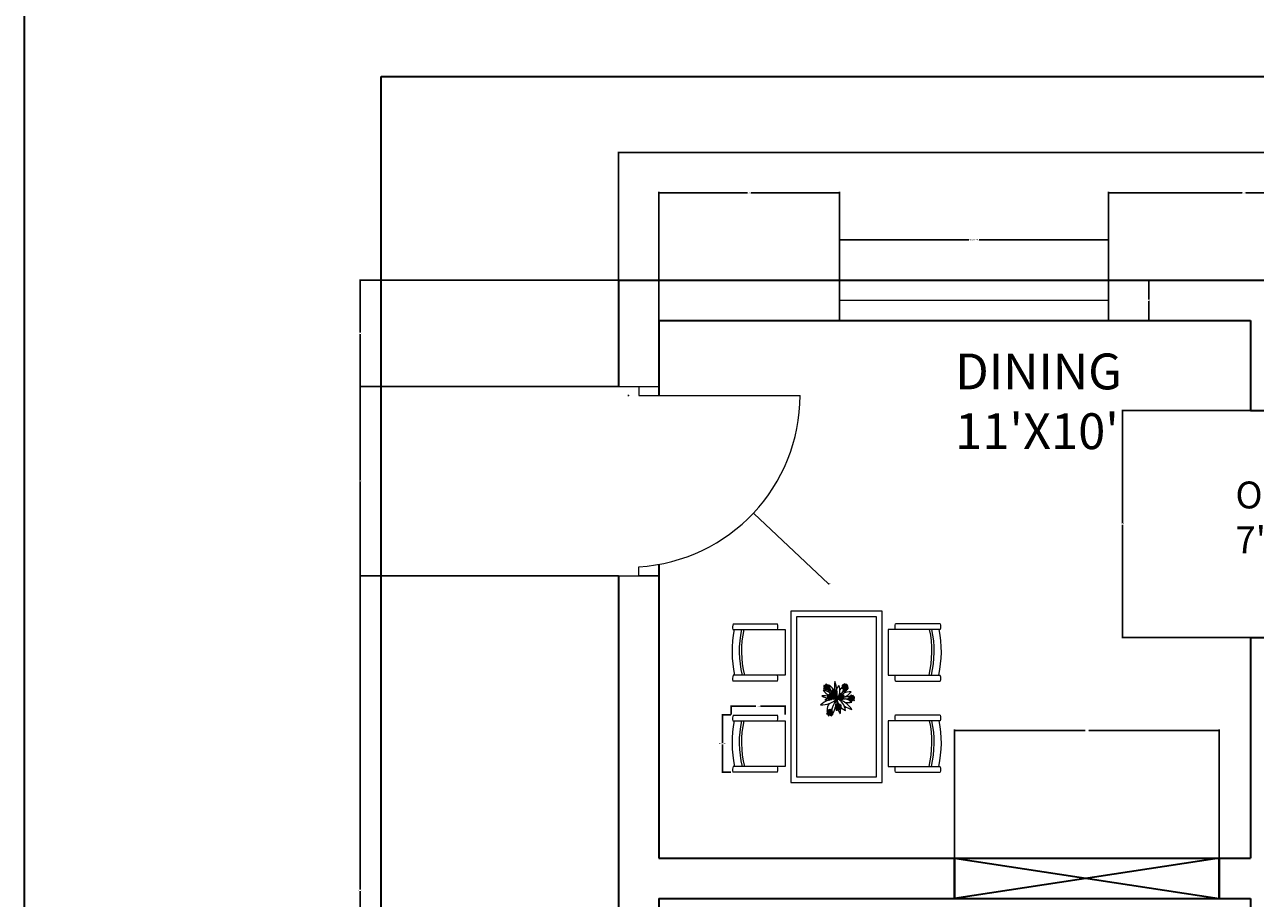
# Model space of a CAD drawing. Units: inches. Extents: x 1976 to 2558, y -977 to 2909.
# Tile 5 of 8: x 1976 to 2251, y 2245 to 2441. Entities that reach past the tile are written whole.
import ezdxf

# ---------------------------------------------------------------- set-up
doc = ezdxf.new("R2010")
doc.units = ezdxf.units.IN
for name, color, linetype, lineweight in [('A-ANNO-DIMS', 2, 'Continuous', 18), ('A-ANNO-TTLB', 7, 'Continuous', 35), ('A-AREA-IDEN', 7, 'Continuous', 18), ('A-DOOR', 3, 'Continuous', 18), ('A-FURN', 8, 'Continuous', 13), ('A-GLAZ', 4, 'Continuous', 18), ('A-WALL', 7, 'Continuous', 35)]:
    doc.layers.add(name, color=color, linetype=linetype, lineweight=lineweight)
doc.styles.get("Standard").update_dxf_attribs({"font": 'arial.ttf'})
doc.dimstyles.get("Standard").update_dxf_attribs({"dimtxt": 0.18, "dimasz": 0.18, "dimexe": 0.18, "dimexo": 0.0625, "dimgap": 0.09, "dimtad": 0, "dimtih": 1, "dimtoh": 1, "dimdec": 4, "dimzin": 0, "dimdsep": 46, "dimtxsty": 'Standard', "dimcen": 0.09, "dimadec": 0, "dimazin": 0, "dimtfac": 1, "dimtdec": 4, "dimtofl": 0, "dimtmove": 0, "dimatfit": 3, "dimfxl": 1, "dimtolj": 1, "dimtzin": 0, "dimarcsym": 0})

# ---------------------------------------------------------------- blocks, each defined once
blk = doc.blocks.new('CHAIR-DINING')
for p, q in [((0.21, 11.47), (11.84, 11.47)), ((0.23, 12.75), (10.16, 12.75)), ((11.84, 11.47), (11.84, 1.28)), ((10.17, 0), (0.21, 0)), ((11.84, 1.28), (0.23, 1.28))]:
    blk.add_line(p, q)
for centre, radius, start, end in [((25.08, 6.69), 25.08, 168.9982, 192.4562), ((2.1, 12.08), 1.98, 160.4535, 197.9116), ((25.42, 6.69), 23.81, 168.4012, 193.1346), ((25.42, 6.69), 23.3, 168.1438, 193.4274), ((8.28, 12.1), 1.98, 342.2774, 19.7376), ((2.1, 0.6), 1.98, 160.2624, 197.7226), ((8.28, 0.6), 1.98, 342.2774, 19.7376)]:
    blk.add_arc(centre, radius, start, end)
blk = doc.blocks.new('WIN-60-PLAN')
for p, q in [((4.5, 60), (0, 60)), ((0, 60), (9, 60)), ((4.5, 0), (4.5, 60)), ((0, 0), (9, 0)), ((9, 0), (4.5, 0))]:
    blk.add_line(p, q)
blk = doc.blocks.new('*D9')
at = {"layer": 'A-ANNO-DIMS', "color": 0, "lineweight": -2, "transparency": 16777216}
for p, q in [((2133.49, 2286.43), (2131.45, 2286.43)), ((2131.63, 2286.25), (2131.63, 2280.23)), ((2131.63, 2273.84), (2131.63, 2279.86)), ((2133.49, 2273.66), (2131.45, 2273.66))]:
    blk.add_line(p, q, dxfattribs=at)
at = {"layer": 'A-ANNO-DIMS', "color": 0, "transparency": 16777216}
for points in [[(2131.6, 2286.25), (2131.66, 2286.25), (2131.63, 2286.43)], [(2131.6, 2273.84), (2131.66, 2273.84), (2131.63, 2273.66)]]:
    blk.add_solid(points, dxfattribs=at)
at = {"layer": 'Defpoints', "color": 0, "transparency": 16777216}
for p in [(2131.63, 2286.43), (2133.55, 2286.43), (2133.55, 2273.66)]:
    blk.add_point(p, dxfattribs=at)
at = {"layer": 'A-ANNO-DIMS', "color": 0, "transparency": 16777216, "insert": (2131.63, 2280.05), "char_height": 0.18, "attachment_point": 5}
blk.add_mtext('\\A1;CHAIR 13 TYP.', dxfattribs=at)
blk = doc.blocks.new('*D10')
at = {"layer": 'A-ANNO-DIMS', "color": 0, "lineweight": -2, "transparency": 16777216}
for p, q in [((2133.55, 2286.49), (2133.55, 2288.53)), ((2133.73, 2288.35), (2139.05, 2288.35)), ((2145.4, 2288.35), (2140.09, 2288.35)), ((2145.58, 2286.49), (2145.58, 2288.53))]:
    blk.add_line(p, q, dxfattribs=at)
at = {"layer": 'A-ANNO-DIMS', "color": 0, "transparency": 16777216}
for points in [[(2133.73, 2288.38), (2133.73, 2288.32), (2133.55, 2288.35)], [(2145.4, 2288.38), (2145.4, 2288.32), (2145.58, 2288.35)]]:
    blk.add_solid(points, dxfattribs=at)
at = {"layer": 'Defpoints', "color": 0, "transparency": 16777216}
for p in [(2145.58, 2288.35), (2133.55, 2286.43), (2145.58, 2286.43)]:
    blk.add_point(p, dxfattribs=at)
at = {"layer": 'A-ANNO-DIMS', "color": 0, "transparency": 16777216, "insert": (2139.57, 2288.35), "char_height": 0.18, "attachment_point": 5}
blk.add_mtext('\\A1;12 TYP.', dxfattribs=at)
blk = doc.blocks.new('*D11')
at = {"layer": 'A-ANNO-DIMS', "color": 0, "lineweight": -2, "transparency": 16777216}
for p, q in [((2157.76, 2383.54), (2157.76, 2392.66)), ((2157.94, 2392.48), (2186.64, 2392.48)), ((2217.58, 2392.48), (2188.88, 2392.48)), ((2217.76, 2383.54), (2217.76, 2392.66))]:
    blk.add_line(p, q, dxfattribs=at)
at = {"layer": 'A-ANNO-DIMS', "color": 0, "transparency": 16777216}
for points in [[(2157.94, 2392.51), (2157.94, 2392.45), (2157.76, 2392.48)], [(2217.58, 2392.51), (2217.58, 2392.45), (2217.76, 2392.48)]]:
    blk.add_solid(points, dxfattribs=at)
at = {"layer": 'Defpoints', "color": 0, "transparency": 16777216}
for p in [(2217.76, 2392.48), (2157.76, 2383.48), (2217.76, 2383.48)]:
    blk.add_point(p, dxfattribs=at)
at = {"layer": 'A-ANNO-DIMS', "color": 0, "transparency": 16777216, "insert": (2187.76, 2392.48), "char_height": 0.18, "attachment_point": 5}
blk.add_mtext('\\A1;WINDOW 60 TYP.', dxfattribs=at)
blk = doc.blocks.new('*D12')
at = {"layer": 'A-ANNO-DIMS', "color": 0, "lineweight": -2, "transparency": 16777216}
for p, q in [((2217.82, 2383.48), (2226.94, 2383.48)), ((2226.76, 2383.3), (2226.76, 2379.16)), ((2226.76, 2374.66), (2226.76, 2378.8)), ((2217.82, 2374.48), (2226.94, 2374.48))]:
    blk.add_line(p, q, dxfattribs=at)
at = {"layer": 'A-ANNO-DIMS', "color": 0, "transparency": 16777216}
for points in [[(2226.73, 2383.3), (2226.79, 2383.3), (2226.76, 2383.48)], [(2226.73, 2374.66), (2226.79, 2374.66), (2226.76, 2374.48)]]:
    blk.add_solid(points, dxfattribs=at)
at = {"layer": 'Defpoints', "color": 0, "transparency": 16777216}
for p in [(2217.76, 2383.48), (2217.76, 2374.48), (2226.76, 2374.48)]:
    blk.add_point(p, dxfattribs=at)
at = {"layer": 'A-ANNO-DIMS', "color": 0, "transparency": 16777216, "insert": (2226.76, 2378.98), "char_height": 0.18, "attachment_point": 5}
blk.add_mtext('\\A1;9 TYP.', dxfattribs=at)
blk = doc.blocks.new('*D23')
at = {"layer": 'A-ANNO-DIMS', "color": 0, "lineweight": -2, "transparency": 16777216}
for p, q in [((2108.44, 2383.54), (2108.44, 2412.16)), ((2108.62, 2411.98), (2256.65, 2411.98)), ((2405.26, 2411.98), (2257.23, 2411.98)), ((2405.44, 2383.54), (2405.44, 2412.16))]:
    blk.add_line(p, q, dxfattribs=at)
at = {"layer": 'A-ANNO-DIMS', "color": 0, "transparency": 16777216}
for points in [[(2108.62, 2412.01), (2108.62, 2411.95), (2108.44, 2411.98)], [(2405.26, 2412.01), (2405.26, 2411.95), (2405.44, 2411.98)]]:
    blk.add_solid(points, dxfattribs=at)
at = {"layer": 'Defpoints', "color": 0, "transparency": 16777216}
for p in [(2405.44, 2411.98), (2108.44, 2383.48), (2405.44, 2383.48)]:
    blk.add_point(p, dxfattribs=at)
at = {"layer": 'A-ANNO-DIMS', "color": 0, "transparency": 16777216, "insert": (2256.94, 2411.98), "char_height": 0.18, "attachment_point": 5}
blk.add_mtext('\\A1;297', dxfattribs=at)
blk = doc.blocks.new('*D28')
at = {"layer": 'A-ANNO-DIMS', "color": 0, "lineweight": -2, "transparency": 16777216}
for p, q in [((2117.44, 2374.54), (2117.44, 2403.16)), ((2117.62, 2402.98), (2137.2, 2402.98)), ((2157.58, 2402.98), (2137.99, 2402.98)), ((2157.76, 2374.54), (2157.76, 2403.16))]:
    blk.add_line(p, q, dxfattribs=at)
at = {"layer": 'A-ANNO-DIMS', "color": 0, "transparency": 16777216}
for points in [[(2117.62, 2403.01), (2117.62, 2402.95), (2117.44, 2402.98)], [(2157.58, 2403.01), (2157.58, 2402.95), (2157.76, 2402.98)]]:
    blk.add_solid(points, dxfattribs=at)
at = {"layer": 'Defpoints', "color": 0, "transparency": 16777216}
for p in [(2157.76, 2402.98), (2117.44, 2374.48), (2157.76, 2374.48)]:
    blk.add_point(p, dxfattribs=at)
at = {"layer": 'A-ANNO-DIMS', "color": 0, "transparency": 16777216, "insert": (2137.6, 2402.98), "char_height": 0.18, "attachment_point": 5}
blk.add_mtext('\\A1;40.32', dxfattribs=at)
blk = doc.blocks.new('*D29')
at = {"layer": 'A-ANNO-DIMS', "color": 0, "lineweight": -2, "transparency": 16777216}
for p, q in [((2217.76, 2374.54), (2217.76, 2403.16)), ((2217.94, 2402.98), (2247.63, 2402.98)), ((2278.11, 2402.98), (2248.42, 2402.98)), ((2278.29, 2374.54), (2278.29, 2403.16))]:
    blk.add_line(p, q, dxfattribs=at)
at = {"layer": 'A-ANNO-DIMS', "color": 0, "transparency": 16777216}
for points in [[(2217.94, 2403.01), (2217.94, 2402.95), (2217.76, 2402.98)], [(2278.11, 2403.01), (2278.11, 2402.95), (2278.29, 2402.98)]]:
    blk.add_solid(points, dxfattribs=at)
at = {"layer": 'Defpoints', "color": 0, "transparency": 16777216}
for p in [(2278.29, 2402.98), (2217.76, 2374.48), (2278.29, 2374.48)]:
    blk.add_point(p, dxfattribs=at)
at = {"layer": 'A-ANNO-DIMS', "color": 0, "transparency": 16777216, "insert": (2248.02, 2402.98), "char_height": 0.18, "attachment_point": 5}
blk.add_mtext('\\A1;60.53', dxfattribs=at)
blk = doc.blocks.new('*D33')
at = {"layer": 'A-ANNO-DIMS', "color": 0, "lineweight": -2, "transparency": 16777216}
for p, q in [((2108.38, 2383.48), (2050.58, 2383.48)), ((2050.76, 2383.3), (2050.76, 2371.8)), ((2050.76, 2359.93), (2050.76, 2371.43)), ((2108.38, 2359.75), (2050.58, 2359.75))]:
    blk.add_line(p, q, dxfattribs=at)
at = {"layer": 'A-ANNO-DIMS', "color": 0, "transparency": 16777216}
for points in [[(2050.73, 2383.3), (2050.79, 2383.3), (2050.76, 2383.48)], [(2050.73, 2359.93), (2050.79, 2359.93), (2050.76, 2359.75)]]:
    blk.add_solid(points, dxfattribs=at)
at = {"layer": 'Defpoints', "color": 0, "transparency": 16777216}
for p in [(2108.44, 2383.48), (2050.76, 2359.75), (2108.44, 2359.75)]:
    blk.add_point(p, dxfattribs=at)
at = {"layer": 'A-ANNO-DIMS', "color": 0, "transparency": 16777216, "insert": (2050.76, 2371.61), "char_height": 0.18, "attachment_point": 5}
blk.add_mtext('\\A1;23.73', dxfattribs=at)
blk = doc.blocks.new('*D34')
at = {"layer": 'A-ANNO-DIMS', "color": 0, "lineweight": -2, "transparency": 16777216}
for p, q in [((2108.38, 2359.75), (2050.58, 2359.75)), ((2050.76, 2359.57), (2050.76, 2338.8)), ((2050.76, 2317.68), (2050.76, 2338.44)), ((2108.38, 2317.5), (2050.58, 2317.5))]:
    blk.add_line(p, q, dxfattribs=at)
at = {"layer": 'A-ANNO-DIMS', "color": 0, "transparency": 16777216}
for points in [[(2050.73, 2359.57), (2050.79, 2359.57), (2050.76, 2359.75)], [(2050.73, 2317.68), (2050.79, 2317.68), (2050.76, 2317.5)]]:
    blk.add_solid(points, dxfattribs=at)
at = {"layer": 'Defpoints', "color": 0, "transparency": 16777216}
for p in [(2108.44, 2359.75), (2050.76, 2317.5), (2108.44, 2317.5)]:
    blk.add_point(p, dxfattribs=at)
at = {"layer": 'A-ANNO-DIMS', "color": 0, "transparency": 16777216, "insert": (2050.76, 2338.62), "char_height": 0.18, "attachment_point": 5}
blk.add_mtext('\\A1;42.25', dxfattribs=at)
blk = doc.blocks.new('*D35')
at = {"layer": 'A-ANNO-DIMS', "color": 0, "lineweight": -2, "transparency": 16777216}
for p, q in [((2108.38, 2317.5), (2050.58, 2317.5)), ((2050.76, 2317.32), (2050.76, 2247.46)), ((2050.76, 2177.24), (2050.76, 2247.1)), ((2108.38, 2177.06), (2050.58, 2177.06))]:
    blk.add_line(p, q, dxfattribs=at)
at = {"layer": 'A-ANNO-DIMS', "color": 0, "transparency": 16777216}
for points in [[(2050.73, 2317.32), (2050.79, 2317.32), (2050.76, 2317.5)], [(2050.73, 2177.24), (2050.79, 2177.24), (2050.76, 2177.06)]]:
    blk.add_solid(points, dxfattribs=at)
at = {"layer": 'Defpoints', "color": 0, "transparency": 16777216}
for p in [(2108.44, 2317.5), (2050.76, 2177.06), (2108.44, 2177.06)]:
    blk.add_point(p, dxfattribs=at)
at = {"layer": 'A-ANNO-DIMS', "color": 0, "transparency": 16777216, "insert": (2050.76, 2247.28), "char_height": 0.18, "attachment_point": 5}
blk.add_mtext('\\A1;140.44', dxfattribs=at)
blk = doc.blocks.new('*D49')
at = {"layer": 'A-ANNO-DIMS', "color": 0, "lineweight": -2, "transparency": 16777216}
for p, q in [((2249.38, 2354.4), (2220.76, 2354.4)), ((2220.94, 2354.22), (2220.94, 2329.25)), ((2220.94, 2303.92), (2220.94, 2328.89)), ((2249.38, 2303.74), (2220.76, 2303.74))]:
    blk.add_line(p, q, dxfattribs=at)
at = {"layer": 'A-ANNO-DIMS', "color": 0, "transparency": 16777216}
for points in [[(2220.91, 2354.22), (2220.97, 2354.22), (2220.94, 2354.4)], [(2220.91, 2303.92), (2220.97, 2303.92), (2220.94, 2303.74)]]:
    blk.add_solid(points, dxfattribs=at)
at = {"layer": 'Defpoints', "color": 0, "transparency": 16777216}
for p in [(2220.94, 2354.4), (2249.44, 2354.4), (2249.44, 2303.74)]:
    blk.add_point(p, dxfattribs=at)
at = {"layer": 'A-ANNO-DIMS', "color": 0, "transparency": 16777216, "insert": (2220.94, 2329.07), "char_height": 0.18, "attachment_point": 5}
blk.add_mtext('\\A1;50.67', dxfattribs=at)
blk = doc.blocks.new('*D50')
at = {"layer": 'A-ANNO-DIMS', "color": 0, "lineweight": -2, "transparency": 16777216}
for p, q in [((2183.44, 2254.54), (2183.44, 2283.16)), ((2183.62, 2282.98), (2212.58, 2282.98)), ((2242.33, 2282.98), (2213.37, 2282.98)), ((2242.51, 2254.54), (2242.51, 2283.16))]:
    blk.add_line(p, q, dxfattribs=at)
at = {"layer": 'A-ANNO-DIMS', "color": 0, "transparency": 16777216}
for points in [[(2183.62, 2283.01), (2183.62, 2282.95), (2183.44, 2282.98)], [(2242.33, 2283.01), (2242.33, 2282.95), (2242.51, 2282.98)]]:
    blk.add_solid(points, dxfattribs=at)
at = {"layer": 'Defpoints', "color": 0, "transparency": 16777216}
for p in [(2242.51, 2282.98), (2183.44, 2254.48), (2242.51, 2254.48)]:
    blk.add_point(p, dxfattribs=at)
at = {"layer": 'A-ANNO-DIMS', "color": 0, "transparency": 16777216, "insert": (2212.97, 2282.98), "char_height": 0.18, "attachment_point": 5}
blk.add_mtext('\\A1;59.07', dxfattribs=at)
blk = doc.blocks.new('*D89')
at = {"layer": 'A-ANNO-DIMS', "color": 0, "lineweight": -2, "transparency": 16777216}
for p, q in [((2110.53, 2357.75), (2110.71, 2357.75)), ((2110.62, 2357.66), (2110.62, 2357.84)), ((2155.27, 2315.73), (2138.65, 2331.36)), ((2155.45, 2315.73), (2155.27, 2315.73))]:
    blk.add_line(p, q, dxfattribs=at)
at = {"layer": 'A-ANNO-DIMS', "color": 0, "transparency": 16777216}
blk.add_solid([(2138.67, 2331.38), (2138.63, 2331.34), (2138.52, 2331.48)], dxfattribs=at)
at = {"layer": 'Defpoints', "color": 0, "transparency": 16777216}
for p in [(2110.62, 2357.75), (2138.52, 2331.48)]:
    blk.add_point(p, dxfattribs=at)
at = {"layer": 'A-ANNO-DIMS', "color": 0, "transparency": 16777216, "insert": (2155.92, 2315.73), "char_height": 0.18, "attachment_point": 5}
blk.add_mtext('\\A1;R38.32', dxfattribs=at)

msp = doc.modelspace()

# ---------------------------------------------------------------- linework, layer by layer
at = {"layer": 'A-ANNO-TTLB'}
for points in [[(1975.8545, 2909.3429), (2557.9168, 2909.3429), (2557.9168, 1747.8598), (1975.8545, 1747.8598)], [(2055.4343, 2428.9091), (2450.0007, 2428.9091), (2450.0007, 1815.3916), (2055.4343, 1815.3916)]]:
    msp.add_lwpolyline(points, close=True, dxfattribs=at)
at = {"layer": 'A-DOOR'}
for p, q in [((2108.4385, 2359.7476), (2117.4385, 2359.7476)), ((2112.9385, 2359.7476), (2112.9385, 2357.7476)), ((2112.9385, 2357.7476), (2148.9385, 2357.7476)), ((2112.9385, 2317.4977), (2112.9385, 2319.4977)), ((2108.4385, 2317.4977), (2117.4385, 2317.4977)), ((2117.4385, 2317.4977), (2112.9385, 2317.4977))]:
    msp.add_line(p, q, dxfattribs=at)
msp.add_arc((2110.6183, 2357.7476), 38.3202, 273.471228, 0, dxfattribs=at)
at = {"layer": 'A-FURN'}
for points in [[(2167.272, 2309.6099), (2146.8785, 2309.6099), (2146.8785, 2271.372), (2167.272, 2271.372)], [(2165.9974, 2308.3353), (2148.1531, 2308.3353), (2148.1531, 2272.6466), (2165.9974, 2272.6466)]]:
    msp.add_lwpolyline(points, close=True, dxfattribs=at)
for centre, radius, start, end in [((2164.1832, 2292.9107), 7.5857, 172.300876, 189.713934), ((2149.6339, 2291.0822), 7.5857, 352.300876, 22.025549), ((2158.1534, 2295.1251), 5.1574, 217.808391, 258.794638), ((2153.0765, 2286.9043), 5.1574, 60.607319, 78.794638), ((2154.169, 2293.3715), 1.0315, 269.156448, 313.437642), ((2154.8631, 2291.5911), 1.0315, 89.156448, 133.437642), ((2154.3081, 2291.3787), 1.3683, 65.373219, 94.46089), ((2154.7718, 2293.9866), 1.3683, 245.373219, 274.46089), ((2155.0787, 2293.6343), 1.0315, 217.808391, 258.794638), ((2154.0633, 2291.9902), 1.0315, 60.607319, 78.794638), ((2154.687, 2291.6856), 0.9563, 78.462149, 111.54354), ((2154.5271, 2293.512), 0.9563, 258.462149, 268.298065), ((2155.632, 2293.808), 1.4049, 211.28949, 237.552058), ((2153.6777, 2291.8929), 1.4049, 31.28949, 57.552058), ((2154.9539, 2292.1195), 0.5087, 145.613299, 182.653681), ((2154.3701, 2292.599), 0.5087, 278.552081, 306.302355), ((2154.0572, 2292.5582), 0.8235, 4.476283, 53.763425), ((2155.3651, 2293.2868), 0.8235, 184.476283, 205.355726), ((2156.0281, 2291.8073), 1.4095, 144.666489, 178.965307), ((2153.469, 2292.648), 1.4095, 324.666489, 343.955925), ((2156.2847, 2293.1915), 1.5171, 172.300876, 189.713934), ((2153.3748, 2292.8258), 1.5171, 352.300876, 22.025549), ((2155.6455, 2292.3211), 0.8243, 158.556067, 197.254243), ((2154.091, 2292.378), 0.8243, 338.556067, 17.254243), ((2155.3702, 2292.8464), 0.5405, 138.054662, 156.71607), ((2154.4763, 2292.9838), 0.5405, 318.054662, 24.46723), ((2153.8722, 2294.2269), 1.8938, 302.089724, 323.743755), ((2156.4053, 2291.5025), 1.8938, 122.089724, 143.743755), ((2155.4004, 2290.8199), 1.8767, 82.537441, 106.153056), ((2155.122, 2294.4833), 1.8767, 262.537441, 286.153056), ((2155.5237, 2292.6892), 0.6489, 185.896009, 246.101931), ((2154.6154, 2292.0293), 0.6489, 5.896009, 66.101931), ((2154.5562, 2291.4603), 1.206, 34.273745, 74.509726), ((2155.8019, 2292.4719), 0.9358, 195.544227, 214.461724), ((2151.1486, 2286.4178), 7.0243, 31.28949, 57.552058), ((2160.9199, 2295.9936), 7.0243, 211.28949, 237.552058), ((2155.6877, 2292.5572), 0.812, 124.966344, 145.814561), ((2154.1067, 2292.093), 0.9358, 350.741507, 11.174689), ((2154.4129, 2293.288), 0.812, 331.307439, 355.385611), ((2155.4951, 2292.1452), 0.7799, 88.595575, 113.612418), ((2155.8748, 2293.3017), 1.206, 236.312373, 254.509726), ((2154.8974, 2293.4022), 0.7799, 293.448679, 322.265702), ((2155.3799, 2293.2756), 0.8235, 258.712866, 281.757983), ((2155.0461, 2291.8162), 0.8235, 52.470844, 74.980876), ((2159.5852, 2293.3872), 4.1177, 184.476283, 205.355726), ((2153.0461, 2289.7446), 4.1177, 4.476283, 53.763425), ((2157.095, 2290.9992), 1.5171, 172.300876, 189.713934), ((2154.1851, 2290.6335), 1.5171, 352.300876, 22.025549), ((2156.4836, 2290.3886), 1.0315, 89.156448, 133.437642), ((2155.7896, 2292.169), 1.0315, 269.156448, 313.437642), ((2155.9287, 2290.1762), 1.3683, 65.373219, 94.46089), ((2156.3924, 2292.7841), 1.3683, 245.373219, 274.46089), ((2155.6839, 2290.7877), 1.0315, 60.607319, 78.794638), ((2156.6993, 2292.4318), 1.0315, 217.808391, 258.794638), ((2156.3076, 2290.483), 0.9563, 78.462149, 111.54354), ((2156.1477, 2292.3094), 0.9563, 258.462149, 268.298065), ((2157.2526, 2292.6055), 1.4049, 211.28949, 237.552058), ((2155.2983, 2290.6903), 1.4049, 31.28949, 57.552058), ((2156.5745, 2290.9169), 0.5087, 145.613299, 182.653681), ((2156.9856, 2292.0842), 0.8235, 184.476283, 205.355726), ((2155.6778, 2291.3557), 0.8235, 4.476283, 53.763425), ((2157.6487, 2290.6048), 1.4095, 144.666489, 178.965307), ((2157.9052, 2291.9889), 1.5171, 172.300876, 189.713934), ((2154.9954, 2291.6232), 1.5171, 352.300876, 22.025549), ((2157.2661, 2291.1186), 0.8243, 158.556067, 197.254243), ((2155.7116, 2291.1755), 0.8243, 338.556067, 17.254243), ((2156.9908, 2291.6438), 0.5405, 138.054662, 156.71607), ((2156.0968, 2291.7813), 0.5405, 318.054662, 24.46723), ((2155.4928, 2293.0244), 1.8938, 302.089724, 323.743755), ((2158.0259, 2290.3), 1.8938, 122.089724, 143.743755), ((2157.0209, 2289.6174), 1.8767, 82.537441, 106.153056), ((2156.7426, 2293.2808), 1.8767, 262.537441, 286.153056), ((2157.1443, 2291.4866), 0.6489, 185.896009, 246.101931), ((2156.236, 2290.8267), 0.6489, 5.896009, 66.101931), ((2156.1767, 2290.2578), 1.206, 34.273745, 74.509726), ((2157.3082, 2291.3546), 0.812, 124.966344, 145.814561), ((2156.0335, 2292.0854), 0.812, 331.307439, 355.385611), ((2157.1157, 2290.9426), 0.7799, 88.595575, 113.612418), ((2157.4954, 2292.0991), 1.206, 236.312373, 254.509726), ((2156.5179, 2292.1997), 0.7799, 293.448679, 322.265702), ((2157.0005, 2292.0731), 0.8235, 258.712866, 281.757983), ((2156.6666, 2290.6137), 0.8235, 52.470844, 74.980876), ((2159.611, 2291.1852), 2.7025, 138.054662, 156.71607), ((2155.1411, 2291.8723), 2.7025, 318.054662, 24.46723), ((2152.1209, 2298.088), 9.4688, 302.089724, 323.743755), ((2164.7866, 2284.4661), 9.4688, 122.089724, 143.743755), ((2157.2984, 2290.4303), 0.8235, 4.476283, 53.763425), ((2158.6062, 2291.1588), 0.8235, 184.476283, 205.355726), ((2161.1982, 2289.7393), 4.0602, 124.966344, 145.814561), ((2159.5258, 2291.0635), 1.5171, 172.300876, 189.713934), ((2156.6159, 2290.6978), 1.5171, 352.300876, 22.025549), ((2158.6114, 2290.7184), 0.5405, 138.054662, 156.71607), ((2157.7174, 2290.8558), 0.5405, 318.054662, 24.46723), ((2158.9145, 2291.6609), 1.0315, 89.156448, 133.437642), ((2158.2205, 2293.4412), 1.0315, 269.156448, 313.437642), ((2158.3595, 2291.4484), 1.3683, 65.373219, 94.46089), ((2158.8233, 2294.0564), 1.3683, 245.373219, 274.46089), ((2158.9288, 2290.4292), 0.812, 124.966344, 145.814561), ((2159.1301, 2293.7041), 1.0315, 217.808391, 258.794638), ((2158.1147, 2292.0599), 1.0315, 60.607319, 78.794638), ((2157.654, 2291.16), 0.812, 331.307439, 355.385611), ((2154.8243, 2293.3932), 4.0602, 331.307439, 355.385611), ((2158.7384, 2291.7553), 0.9563, 78.462149, 111.54354), ((2158.5785, 2293.5817), 0.9563, 258.462149, 268.298065), ((2159.6834, 2293.8778), 1.4049, 211.28949, 237.552058), ((2157.7292, 2291.9626), 1.4049, 31.28949, 57.552058), ((2159.0053, 2292.1892), 0.5087, 145.613299, 182.653681), ((2158.4215, 2292.6687), 0.5087, 278.552081, 306.302355), ((2159.4165, 2293.3565), 0.8235, 184.476283, 205.355726), ((2158.1087, 2292.628), 0.8235, 4.476283, 53.763425), ((2160.0796, 2291.8771), 1.4095, 144.666489, 178.965307), ((2157.5204, 2292.7177), 1.4095, 324.666489, 343.955925), ((2160.2353, 2287.6793), 3.8997, 88.595575, 113.612418), ((2157.2468, 2293.9645), 3.8997, 293.448679, 322.265702), ((2160.3361, 2293.2612), 1.5171, 172.300876, 189.713934), ((2157.4262, 2292.8955), 1.5171, 352.300876, 22.025549), ((2159.6969, 2292.3909), 0.8243, 158.556067, 197.254243), ((2158.1425, 2292.4477), 0.8243, 338.556067, 17.254243), ((2159.4216, 2292.9161), 0.5405, 138.054662, 156.71607), ((2158.5277, 2293.0535), 0.5405, 318.054662, 24.46723), ((2157.9236, 2294.2967), 1.8938, 302.089724, 323.743755), ((2160.4568, 2291.5723), 1.8938, 122.089724, 143.743755), ((2159.4518, 2290.8896), 1.8767, 82.537441, 106.153056), ((2159.1734, 2294.553), 1.8767, 262.537441, 286.153056), ((2159.5751, 2292.7589), 0.6489, 185.896009, 246.101931), ((2158.6668, 2292.099), 0.6489, 5.896009, 66.101931), ((2158.6076, 2291.5301), 1.206, 34.273745, 74.509726), ((2159.8533, 2292.5417), 0.9358, 195.544227, 214.461724), ((2159.7391, 2292.6269), 0.812, 124.966344, 145.814561), ((2158.1581, 2292.1627), 0.9358, 350.741507, 11.174689), ((2158.4643, 2293.3577), 0.812, 331.307439, 355.385611), ((2159.5465, 2292.2149), 0.7799, 88.595575, 113.612418), ((2159.9263, 2293.3714), 1.206, 236.312373, 254.509726), ((2158.9488, 2293.472), 0.7799, 293.448679, 322.265702), ((2159.4314, 2293.3453), 0.8235, 258.712866, 281.757983), ((2159.0975, 2291.886), 0.8235, 52.470844, 74.980876), ((2157.0753, 2284.909), 5.1575, 89.156448, 133.437642), ((2153.6051, 2293.8109), 5.1575, 269.156448, 313.437642), ((2154.3003, 2283.8468), 6.8414, 65.373219, 94.46089), ((2156.6191, 2296.8866), 6.8414, 245.373219, 274.46089), ((2156.1949, 2285.3813), 4.7813, 78.462149, 111.54354), ((2155.3955, 2294.5132), 4.7813, 258.462149, 268.298065), ((2155.6734, 2289.3988), 1.0315, 89.156448, 133.437642), ((2154.9793, 2291.1792), 1.0315, 269.156448, 313.437642), ((2157.5294, 2287.5508), 2.5435, 145.613299, 182.653681), ((2155.1184, 2289.1864), 1.3683, 65.373219, 94.46089), ((2155.5821, 2291.7944), 1.3683, 245.373219, 274.46089), ((2155.889, 2291.4421), 1.0315, 217.808391, 258.794638), ((2154.8736, 2289.7979), 1.0315, 60.607319, 78.794638), ((2155.4973, 2289.4933), 0.9563, 78.462149, 111.54354), ((2155.3374, 2291.3197), 0.9563, 258.462149, 268.298065), ((2156.4423, 2291.6158), 1.4049, 211.28949, 237.552058), ((2154.488, 2289.7006), 1.4049, 31.28949, 57.552058), ((2155.7642, 2289.9272), 0.5087, 145.613299, 182.653681), ((2155.1804, 2290.4067), 0.5087, 278.552081, 306.302355), ((2154.8675, 2290.366), 0.8235, 4.476283, 53.763425), ((2156.1754, 2291.0945), 0.8235, 184.476283, 205.355726), ((2156.8384, 2289.6151), 1.4095, 144.666489, 178.965307), ((2154.2793, 2290.4557), 1.4095, 324.666489, 343.955925), ((2156.4558, 2290.1289), 0.8243, 158.556067, 197.254243), ((2154.9013, 2290.1857), 0.8243, 338.556067, 17.254243), ((2156.1805, 2290.6541), 0.5405, 138.054662, 156.71607), ((2155.2865, 2290.7915), 0.5405, 318.054662, 24.46723), ((2154.6825, 2292.0347), 1.8938, 302.089724, 323.743755), ((2157.2156, 2289.3103), 1.8938, 122.089724, 143.743755), ((2156.2106, 2288.6276), 1.8767, 82.537441, 106.153056), ((2155.9323, 2292.291), 1.8767, 262.537441, 286.153056), ((2156.334, 2290.4969), 0.6489, 185.896009, 246.101931), ((2155.4257, 2289.837), 0.6489, 5.896009, 66.101931), ((2155.3665, 2289.2681), 1.206, 34.273745, 74.509726), ((2156.6122, 2290.2797), 0.9358, 195.544227, 214.461724), ((2156.498, 2290.3649), 0.812, 124.966344, 145.814561), ((2154.917, 2289.9007), 0.9358, 350.741507, 11.174689), ((2162.9006, 2285.9901), 7.0476, 144.666489, 178.965307), ((2155.2232, 2291.0957), 0.812, 331.307439, 355.385611), ((2156.3054, 2289.9529), 0.7799, 88.595575, 113.612418), ((2156.6851, 2291.1094), 1.206, 236.312373, 254.509726), ((2155.7077, 2291.2099), 0.7799, 293.448679, 322.265702), ((2156.1902, 2291.0833), 0.8235, 258.712866, 281.757983), ((2155.9907, 2291.3964), 0.5087, 278.552081, 306.302355), ((2155.8564, 2289.624), 0.8235, 52.470844, 74.980876), ((2155.0896, 2291.4454), 1.4095, 324.666489, 343.955925), ((2157.4225, 2291.2694), 0.9358, 195.544227, 214.461724), ((2155.7272, 2290.8904), 0.9358, 350.741507, 11.174689), ((2156.874, 2287.0313), 1.3683, 65.373219, 94.46089), ((2157.3377, 2289.6392), 1.3683, 245.373219, 274.46089), ((2156.6292, 2287.6428), 1.0315, 60.607319, 78.794638), ((2157.6446, 2289.2869), 1.0315, 217.808391, 258.794638), ((2160.9874, 2288.5591), 4.1216, 158.556067, 197.254243), ((2158.1979, 2289.4606), 1.4049, 211.28949, 237.552058), ((2156.2436, 2287.5455), 1.4049, 31.28949, 57.552058), ((2153.2151, 2288.8434), 4.1216, 338.556067, 17.254243), ((2156.6231, 2288.2108), 0.8235, 4.476283, 53.763425), ((2157.931, 2288.9394), 0.8235, 184.476283, 205.355726), ((2159.7617, 2281.053), 9.3834, 82.537441, 106.153056), ((2158.3699, 2299.3699), 9.3834, 262.537441, 286.153056), ((2160.3784, 2290.3992), 3.2443, 185.896009, 246.101931), ((2155.8369, 2287.0997), 3.2443, 5.896009, 66.101931), ((2155.5407, 2284.2551), 6.0299, 34.273745, 74.509726), ((2158.8506, 2288.8441), 1.5171, 172.300876, 189.713934), ((2155.9407, 2288.4784), 1.5171, 352.300876, 22.025549), ((2158.1042, 2289.4631), 1.0315, 89.156448, 133.437642), ((2157.4102, 2291.2435), 1.0315, 269.156448, 313.437642), ((2157.9361, 2288.499), 0.5405, 138.054662, 156.71607), ((2157.5492, 2289.2507), 1.3683, 65.373219, 94.46089), ((2158.013, 2291.8587), 1.3683, 245.373219, 274.46089), ((2157.0422, 2288.6364), 0.5405, 318.054662, 24.46723), ((2156.4381, 2289.8795), 1.8938, 302.089724, 323.743755), ((2158.9712, 2287.1551), 1.8938, 122.089724, 143.743755), ((2157.9663, 2286.4725), 1.8767, 82.537441, 106.153056), ((2157.6879, 2290.1359), 1.8767, 262.537441, 286.153056), ((2158.3198, 2291.5064), 1.0315, 217.808391, 258.794638), ((2157.3045, 2289.8622), 1.0315, 60.607319, 78.794638), ((2157.9281, 2289.5576), 0.9563, 78.462149, 111.54354), ((2157.7683, 2291.384), 0.9563, 258.462149, 268.298065), ((2158.2536, 2288.2098), 0.812, 124.966344, 145.814561), ((2158.8731, 2291.6801), 1.4049, 211.28949, 237.552058), ((2156.9189, 2289.7649), 1.4049, 31.28949, 57.552058), ((2158.195, 2289.9915), 0.5087, 145.613299, 182.653681), ((2157.6113, 2290.471), 0.5087, 278.552081, 306.302355), ((2156.9788, 2288.9406), 0.812, 331.307439, 355.385611), ((2158.061, 2287.7978), 0.7799, 88.595575, 113.612418), ((2157.4633, 2289.0548), 0.7799, 293.448679, 322.265702), ((2159.2693, 2289.6794), 1.4095, 144.666489, 178.965307), ((2156.7101, 2290.52), 1.4095, 324.666489, 343.955925), ((2158.8867, 2290.1932), 0.8243, 158.556067, 197.254243), ((2157.3322, 2290.25), 0.8243, 338.556067, 17.254243), ((2159.6465, 2289.3746), 1.8938, 122.089724, 143.743755), ((2157.1134, 2292.099), 1.8938, 302.089724, 323.743755), ((2158.6415, 2288.6919), 1.8767, 82.537441, 106.153056), ((2158.3631, 2292.3553), 1.8767, 262.537441, 286.153056), ((2157.7973, 2289.3324), 1.206, 34.273745, 74.509726), ((2158.7648, 2290.5612), 0.6489, 185.896009, 246.101931), ((2157.8565, 2289.9013), 0.6489, 5.896009, 66.101931), ((2159.043, 2290.344), 0.9358, 195.544227, 214.461724), ((2157.3478, 2289.965), 0.9358, 350.741507, 11.174689), ((2158.7362, 2290.0172), 0.7799, 88.595575, 113.612418), ((2159.116, 2291.1737), 1.206, 236.312373, 254.509726), ((2158.1385, 2291.2742), 0.7799, 293.448679, 322.265702), ((2158.6211, 2291.1476), 0.8235, 258.712866, 281.757983), ((2158.2872, 2289.6883), 0.8235, 52.470844, 74.980876), ((2162.134, 2293.4617), 6.0299, 236.312373, 254.509726), ((2159.6595, 2293.3315), 4.1177, 258.712866, 281.757983), ((2157.9903, 2286.0347), 4.1177, 52.470844, 74.980876), ((2160.4, 2289.129), 1.0315, 89.156448, 133.437642), ((2159.706, 2290.9094), 1.0315, 269.156448, 313.437642), ((2159.845, 2288.9166), 1.3683, 65.373219, 94.46089), ((2160.3088, 2291.5245), 1.3683, 245.373219, 274.46089), ((2160.6157, 2291.1722), 1.0315, 217.808391, 258.794638), ((2159.6003, 2289.5281), 1.0315, 60.607319, 78.794638), ((2160.2239, 2289.2235), 0.9563, 78.462149, 111.54354), ((2160.0641, 2291.0498), 0.9563, 258.462149, 268.298065), ((2159.2147, 2289.4308), 1.4049, 31.28949, 57.552058), ((2161.169, 2291.3459), 1.4049, 211.28949, 237.552058), ((2160.4909, 2289.6574), 0.5087, 145.613299, 182.653681), ((2159.9071, 2290.1368), 0.5087, 278.552081, 306.302355), ((2159.5942, 2290.0961), 0.8235, 4.476283, 53.763425), ((2160.902, 2290.8246), 0.8235, 184.476283, 205.355726), ((2161.5651, 2289.3452), 1.4095, 144.666489, 178.965307), ((2159.0059, 2290.1858), 1.4095, 324.666489, 343.955925), ((2161.8216, 2290.7293), 1.5171, 172.300876, 189.713934), ((2158.9118, 2290.3636), 1.5171, 352.300876, 22.025549), ((2161.1825, 2289.859), 0.8243, 158.556067, 197.254243), ((2159.628, 2289.9159), 0.8243, 338.556067, 17.254243), ((2160.9072, 2290.3842), 0.5405, 138.054662, 156.71607), ((2160.0132, 2290.5217), 0.5405, 318.054662, 24.46723), ((2161.9423, 2289.0404), 1.8938, 122.089724, 143.743755), ((2159.4092, 2291.7648), 1.8938, 302.089724, 323.743755), ((2160.9373, 2288.3578), 1.8767, 82.537441, 106.153056), ((2160.6589, 2292.0212), 1.8767, 262.537441, 286.153056), ((2161.0606, 2290.227), 0.6489, 185.896009, 246.101931), ((2160.1523, 2289.5671), 0.6489, 5.896009, 66.101931), ((2160.0931, 2288.9982), 1.206, 34.273745, 74.509726), ((2161.3388, 2290.0098), 0.9358, 195.544227, 214.461724), ((2161.2246, 2290.0951), 0.812, 124.966344, 145.814561), ((2159.6436, 2289.6309), 0.9358, 350.741507, 11.174689), ((2159.9498, 2290.8258), 0.812, 331.307439, 355.385611), ((2161.032, 2289.6831), 0.7799, 88.595575, 113.612418), ((2161.4118, 2290.8395), 1.206, 236.312373, 254.509726), ((2160.4343, 2290.9401), 0.7799, 293.448679, 322.265702), ((2160.9169, 2290.8135), 0.8235, 258.712866, 281.757983), ((2160.583, 2289.3541), 0.8235, 52.470844, 74.980876), ((2155.5383, 2285.9243), 1.0315, 89.156448, 133.437642), ((2154.8443, 2287.7047), 1.0315, 269.156448, 313.437642), ((2154.9833, 2285.7119), 1.3683, 65.373219, 94.46089), ((2155.4471, 2288.3199), 1.3683, 245.373219, 274.46089), ((2155.7539, 2287.9676), 1.0315, 217.808391, 258.794638), ((2154.7386, 2286.3234), 1.0315, 60.607319, 78.794638), ((2154.6105, 2289.9482), 2.5435, 278.552081, 306.302355), ((2155.3622, 2286.0188), 0.9563, 78.462149, 111.54354), ((2155.2024, 2287.8452), 0.9563, 258.462149, 268.298065), ((2156.3072, 2288.1413), 1.4049, 211.28949, 237.552058), ((2154.353, 2286.2261), 1.4049, 31.28949, 57.552058), ((2155.6291, 2286.4527), 0.5087, 145.613299, 182.653681), ((2155.0454, 2286.9322), 0.5087, 278.552081, 306.302355), ((2154.7325, 2286.8915), 0.8235, 4.476283, 53.763425), ((2156.0403, 2287.62), 0.8235, 184.476283, 205.355726), ((2156.7034, 2286.1406), 1.4095, 144.666489, 178.965307), ((2154.1442, 2286.9812), 1.4095, 324.666489, 343.955925), ((2156.9599, 2287.5247), 1.5171, 172.300876, 189.713934), ((2154.05, 2287.159), 1.5171, 352.300876, 22.025549), ((2156.3208, 2286.6544), 0.8243, 158.556067, 197.254243), ((2154.7663, 2286.7112), 0.8243, 338.556067, 17.254243), ((2156.0455, 2287.1796), 0.5405, 138.054662, 156.71607), ((2155.1515, 2287.317), 0.5405, 318.054662, 24.46723), ((2154.5474, 2288.5602), 1.8938, 302.089724, 323.743755), ((2157.0806, 2285.8358), 1.8938, 122.089724, 143.743755), ((2156.0756, 2285.1531), 1.8767, 82.537441, 106.153056), ((2155.7972, 2288.8165), 1.8767, 262.537441, 286.153056), ((2155.2314, 2285.7936), 1.206, 34.273745, 74.509726), ((2156.1989, 2287.0224), 0.6489, 185.896009, 246.101931), ((2155.2906, 2286.3625), 0.6489, 5.896009, 66.101931), ((2156.4771, 2286.8052), 0.9358, 195.544227, 214.461724), ((2156.3629, 2286.8904), 0.812, 124.966344, 145.814561), ((2154.7819, 2286.4262), 0.9358, 350.741507, 11.174689), ((2155.0881, 2287.6212), 0.812, 331.307439, 355.385611), ((2150.1048, 2290.1932), 7.0476, 324.666489, 343.955925), ((2156.1703, 2286.4784), 0.7799, 88.595575, 113.612418), ((2156.5501, 2287.6349), 1.206, 236.312373, 254.509726), ((2155.5726, 2287.7355), 0.7799, 293.448679, 322.265702), ((2156.0552, 2287.6088), 0.8235, 258.712866, 281.757983), ((2155.7213, 2286.1495), 0.8235, 52.470844, 74.980876), ((2157.429, 2287.2437), 1.0315, 89.156448, 133.437642), ((2156.7349, 2289.0241), 1.0315, 269.156448, 313.437642), ((2157.2529, 2287.3382), 0.9563, 78.462149, 111.54354), ((2157.093, 2289.1646), 0.9563, 258.462149, 268.298065), ((2157.5198, 2287.7721), 0.5087, 145.613299, 182.653681), ((2156.936, 2288.2516), 0.5087, 278.552081, 306.302355), ((2158.594, 2287.4599), 1.4095, 144.666489, 178.965307), ((2156.0349, 2288.3006), 1.4095, 324.666489, 343.955925), ((2161.7693, 2289.3131), 4.6791, 195.544227, 214.461724), ((2158.2114, 2287.9737), 0.8243, 158.556067, 197.254243), ((2156.6569, 2288.0306), 0.8243, 338.556067, 17.254243), ((2158.0896, 2288.3418), 0.6489, 185.896009, 246.101931), ((2157.1813, 2287.6819), 0.6489, 5.896009, 66.101931), ((2157.1221, 2287.1129), 1.206, 34.273745, 74.509726), ((2158.3678, 2288.1245), 0.9358, 195.544227, 214.461724), ((2156.6726, 2287.7456), 0.9358, 350.741507, 11.174689), ((2158.4407, 2288.9543), 1.206, 236.312373, 254.509726), ((2157.9458, 2288.9282), 0.8235, 258.712866, 281.757983), ((2157.612, 2287.4688), 0.8235, 52.470844, 74.980876), ((2153.2933, 2287.4183), 4.6791, 350.741507, 11.174689)]:
    msp.add_arc(centre, radius, start, end, dxfattribs=at)
at = {"layer": 'A-WALL'}
for p, q in [((2108.4385, 2383.4789), (2405.4385, 2383.4789)), ((2108.4385, 2383.4789), (2108.4385, 2359.7476)), ((2117.4385, 2374.4789), (2249.4385, 2374.4789)), ((2117.4385, 2374.4789), (2117.4385, 2357.7476)), ((2249.4385, 2374.4789), (2249.4385, 2354.4047)), ((2249.4385, 2354.4047), (2253.9385, 2354.4047)), ((2117.4385, 2320.0392), (2117.4385, 2254.4789)), ((2108.4385, 2317.4977), (2108.4385, 2026.4789)), ((2249.4385, 2303.735), (2253.9385, 2303.735)), ((2249.4385, 2303.735), (2249.4385, 2254.4789)), ((2117.4385, 2254.4789), (2249.4385, 2254.4789)), ((2183.4385, 2254.4789), (2183.4385, 2245.4789)), ((2242.5096, 2254.4789), (2183.4385, 2245.4789)), ((2183.4385, 2245.4789), (2183.4385, 2254.4789)), ((2183.4385, 2254.4789), (2242.5096, 2245.4789)), ((2242.5096, 2254.4789), (2242.5096, 2245.4789)), ((2242.5096, 2245.4789), (2242.5096, 2254.4789)), ((2242.5096, 2254.4789), (2242.5096, 2254.4789)), ((2117.4385, 2245.4789), (2249.4385, 2245.4789)), ((2117.4385, 2245.4789), (2117.4385, 2035.4789)), ((2249.4385, 2245.4789), (2249.4385, 2161.4789))]:
    msp.add_line(p, q, dxfattribs=at)

# ---------------------------------------------------------------- block references
at = {"layer": 'A-FURN'}
for p in [(2133.747, 2294.004), (2133.747, 2273.6605)]:
    msp.add_blockref('CHAIR-DINING', p, dxfattribs=at)
at = {"layer": 'A-FURN', "extrusion": (0, 0, -1), "zscale": -1}
for p in [(-2180.4035, 2294.004), (-2180.4035, 2273.6605)]:
    msp.add_blockref('CHAIR-DINING', p, dxfattribs=at)
at = {"layer": 'A-GLAZ', "rotation": 269.9999999999993}
msp.add_blockref('WIN-60-PLAN', (2157.7586, 2383.4794), dxfattribs=at)

# ---------------------------------------------------------------- texts
at = {"layer": 'A-AREA-IDEN', "attachment_point": 1}
for s, width, insert, char_height in [("DINING\\P11'X10'", 87.726586, (2183.5472, 2367.1042), 8), ('OPEN KITCHEN\\P7\'6"X7\'', 68.564722, (2246.1106, 2338.5313), 6)]:
    msp.add_mtext_dynamic_manual_height_columns(s, width=width, gutter_width=12.5, heights=[0], dxfattribs=dict(at, insert=insert, char_height=char_height))

# ---------------------------------------------------------------- dimensions: what is measured, and where the dimension line sits
at = {"layer": 'A-ANNO-DIMS'}
for base, p1, p2, override, picture, middle in [((2405.4385, 2411.9789), (2108.4385, 2383.4789), (2405.4385, 2383.4789), {"dimdec": 0, "dimlfac": 1, "dimrnd": 0, "dimzin": 0, "dimdsep": 46, "dimlunit": 2}, '*D23', (2256.9385, 2411.9789)), ((2157.7585, 2402.9789), (2117.4385, 2374.4789), (2157.7585, 2374.4789), {"dimdec": 2, "dimlfac": 1, "dimrnd": 0, "dimzin": 0, "dimdsep": 46, "dimlunit": 2}, '*D28', (2137.5985, 2402.9789)), ((2242.5096, 2282.9789), (2183.4385, 2254.4789), (2242.5096, 2254.4789), {"dimdec": 2, "dimlfac": 1, "dimrnd": 0, "dimzin": 0, "dimdsep": 46, "dimlunit": 2}, '*D50', (2212.9741, 2282.9789))]:
    dim = msp.add_linear_dim(base=base, p1=p1, p2=p2, dimstyle='Standard', override=override, dxfattribs=at)
    dim.commit()
    dim.dimension.update_dxf_attribs({"geometry": picture, "text_midpoint": middle})
for base, p1, p2, angle, picture, middle in [((2278.2865, 2402.9789), (2217.7585, 2374.4789), (2278.2865, 2374.4789), 0, '*D29', (2248.0225, 2402.9789)), ((2050.7562, 2359.7476), (2108.4385, 2383.4789), (2108.4385, 2359.7476), 90, '*D33', (2050.7562, 2371.6132)), ((2050.7562, 2317.4977), (2108.4385, 2359.7476), (2108.4385, 2317.4977), 90, '*D34', (2050.7562, 2338.6226)), ((2220.9385, 2354.4047), (2249.4385, 2303.735), (2249.4385, 2354.4047), 90, '*D49', (2220.9385, 2329.0698)), ((2050.7562, 2177.0569), (2108.4385, 2317.4977), (2108.4385, 2177.0569), 90, '*D35', (2050.7562, 2247.2773))]:
    dim = msp.add_linear_dim(base=base, p1=p1, p2=p2, angle=angle, dimstyle='Standard', override={"dimdec": 2, "dimlfac": 1, "dimrnd": 0, "dimzin": 0, "dimdsep": 46, "dimlunit": 2}, dxfattribs=at)
    dim.commit()
    dim.dimension.update_dxf_attribs({"geometry": picture, "text_midpoint": middle})
for base, p1, p2, text, picture, middle in [((2217.7585, 2392.4789), (2157.7585, 2383.4789), (2217.7585, 2383.4789), 'WINDOW <> TYP.', '*D11', (2187.7585, 2392.4789)), ((2145.5843, 2288.3479), (2133.5505, 2286.4321), (2145.5843, 2286.4321), '<> TYP.', '*D10', (2139.5674, 2288.3479))]:
    dim = msp.add_linear_dim(base=base, p1=p1, p2=p2, text=text, dimstyle='Standard', override={"dimdec": 0, "dimlfac": 1, "dimrnd": 0, "dimzin": 0, "dimdsep": 46, "dimlunit": 2}, dxfattribs=at)
    dim.commit()
    dim.dimension.update_dxf_attribs({"geometry": picture, "text_midpoint": middle})
for base, p1, p2, angle, text, picture, middle in [((2226.7585, 2374.4789), (2217.7585, 2383.4789), (2217.7585, 2374.4789), 270, '<> TYP.', '*D12', (2226.7585, 2378.9789)), ((2131.6347, 2286.4321), (2133.5505, 2273.6603), (2133.5505, 2286.4321), 90, 'CHAIR <> TYP.', '*D9', (2131.6347, 2280.0462))]:
    dim = msp.add_linear_dim(base=base, p1=p1, p2=p2, angle=angle, text=text, dimstyle='Standard', override={"dimdec": 0, "dimlfac": 1, "dimrnd": 0, "dimzin": 0, "dimdsep": 46, "dimlunit": 2}, dxfattribs=at)
    dim.commit()
    dim.dimension.update_dxf_attribs({"geometry": picture, "text_midpoint": middle})
dim = msp.add_radius_dim(center=(2110.6183, 2357.7476), mpoint=(2138.5229, 2331.4841), dimstyle='Standard', override={"dimdec": 2, "dimlfac": 1, "dimrnd": 0, "dimzin": 0, "dimdsep": 46, "dimlunit": 2}, dxfattribs=at)
dim.commit()
dim.dimension.update_dxf_attribs({"geometry": '*D89', "text_midpoint": (2155.9246, 2315.726), "dimtype": 164})

doc.saveas('drawing.dxf')
